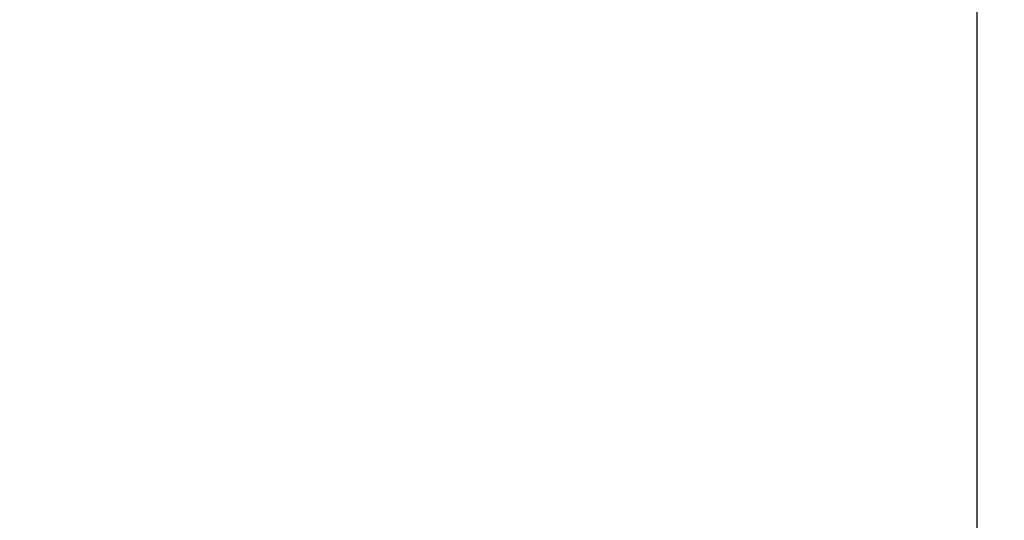
# Model space of a CAD drawing. Units: inches. Extents: x -48 to 50072, y 0 to 21068.
# Tile 31 of 75: x 341 to 467, y 353 to 417. Entities that reach past the tile are written whole.
import ezdxf

# ---------------------------------------------------------------- set-up
doc = ezdxf.new("R2010")
doc.units = ezdxf.units.IN
doc.header["$MEASUREMENT"] = 0
doc.layers.add('A-ANNO-DIMS', color=2, linetype='Continuous', lineweight=18)
doc.styles.get("Standard").update_dxf_attribs({"font": 'arial.ttf'})
doc.dimstyles.get("Standard").update_dxf_attribs({"dimtxt": 8, "dimasz": 0.18, "dimexe": 0.18, "dimexo": 0.0625, "dimgap": 0.09, "dimtad": 0, "dimtih": 1, "dimtoh": 1, "dimdec": 1, "dimzin": 0, "dimdsep": 46, "dimlunit": 4, "dimtxsty": 'Standard', "dimblk": 'ARCHTICK', "dimcen": 0.09, "dimadec": 0, "dimazin": 0, "dimtfac": 1, "dimtdec": 1, "dimtofl": 0, "dimtmove": 0, "dimatfit": 3, "dimldrblk": 'ARCHTICK', "dimfxl": 1, "dimtolj": 1, "dimtzin": 0, "dimarcsym": 0})

# ---------------------------------------------------------------- blocks, each defined once
blk = doc.blocks.new('_ArchTick')
at = {"color": 0, "linetype": 'ByBlock', "const_width": 0.15}
blk.add_lwpolyline([(-0.5, -0.5), (0.5, 0.5)], dxfattribs=at)
blk = doc.blocks.new('*D118')
at = {"layer": 'A-ANNO-DIMS', "color": 0, "lineweight": -2, "transparency": 16777216}
for p, q in [((297.02, 488.71), (297.02, 165.94)), ((463.52, 488.71), (463.52, 165.94)), ((297.02, 166.12), (367.03, 166.12)), ((463.52, 166.12), (393.51, 166.12))]:
    blk.add_line(p, q, dxfattribs=at)
at = {"layer": 'Defpoints', "color": 0, "transparency": 16777216}
for p in [(297.02, 488.77), (463.52, 488.77), (463.52, 166.12)]:
    blk.add_point(p, dxfattribs=at)
at = {"layer": 'A-ANNO-DIMS', "color": 0, "lineweight": -2, "transparency": 16777216, "xscale": 0.18, "yscale": 0.18, "zscale": 0.18, "rotation": 180}
blk.add_blockref('_ArchTick', (297.02, 166.12), dxfattribs=at)
at = {"layer": 'A-ANNO-DIMS', "color": 0, "lineweight": -2, "transparency": 16777216, "xscale": 0.18, "yscale": 0.18, "zscale": 0.18}
blk.add_blockref('_ArchTick', (463.52, 166.12), dxfattribs=at)
at = {"layer": 'A-ANNO-DIMS', "color": 0, "transparency": 16777216, "insert": (380.27, 166.12), "char_height": 8, "attachment_point": 5}
blk.add_mtext('\\A1;166.5', dxfattribs=at)
blk = doc.blocks.new('*D119')
at = {"layer": 'A-ANNO-DIMS', "color": 0, "lineweight": -2, "transparency": 16777216}
for p, q in [((463.52, 451.01), (463.52, 165.94)), ((549.02, 451.01), (549.02, 165.94)), ((463.52, 166.12), (495.75, 166.12)), ((549.02, 166.12), (516.78, 166.12))]:
    blk.add_line(p, q, dxfattribs=at)
at = {"layer": 'Defpoints', "color": 0, "transparency": 16777216}
for p in [(463.52, 451.07), (549.02, 451.07), (549.02, 166.12)]:
    blk.add_point(p, dxfattribs=at)
at = {"layer": 'A-ANNO-DIMS', "color": 0, "lineweight": -2, "transparency": 16777216, "xscale": 0.18, "yscale": 0.18, "zscale": 0.18, "rotation": 180}
blk.add_blockref('_ArchTick', (463.52, 166.12), dxfattribs=at)
at = {"layer": 'A-ANNO-DIMS', "color": 0, "lineweight": -2, "transparency": 16777216, "xscale": 0.18, "yscale": 0.18, "zscale": 0.18}
blk.add_blockref('_ArchTick', (549.02, 166.12), dxfattribs=at)
at = {"layer": 'A-ANNO-DIMS', "color": 0, "transparency": 16777216, "insert": (506.27, 166.12), "char_height": 8, "attachment_point": 5}
blk.add_mtext('\\A1;85.5', dxfattribs=at)

msp = doc.modelspace()

# ---------------------------------------------------------------- dimensions: what is measured, and where the dimension line sits
at = {"layer": 'A-ANNO-DIMS'}
for base, p1, p2, picture, middle in [((463.517, 166.125), (297.017, 488.775), (463.517, 488.775), '*D118', (380.267, 166.125)), ((549.017, 166.125), (463.517, 451.075), (549.017, 451.075), '*D119', (506.267, 166.125))]:
    dim = msp.add_linear_dim(base=base, p1=p1, p2=p2, dimstyle='Standard', override={"dimdec": 1, "dimlfac": 1, "dimrnd": 0, "dimzin": 0, "dimdsep": 46, "dimlunit": 2}, dxfattribs=at)
    dim.commit()
    dim.dimension.update_dxf_attribs({"geometry": picture, "text_midpoint": middle})

doc.saveas('drawing.dxf')
